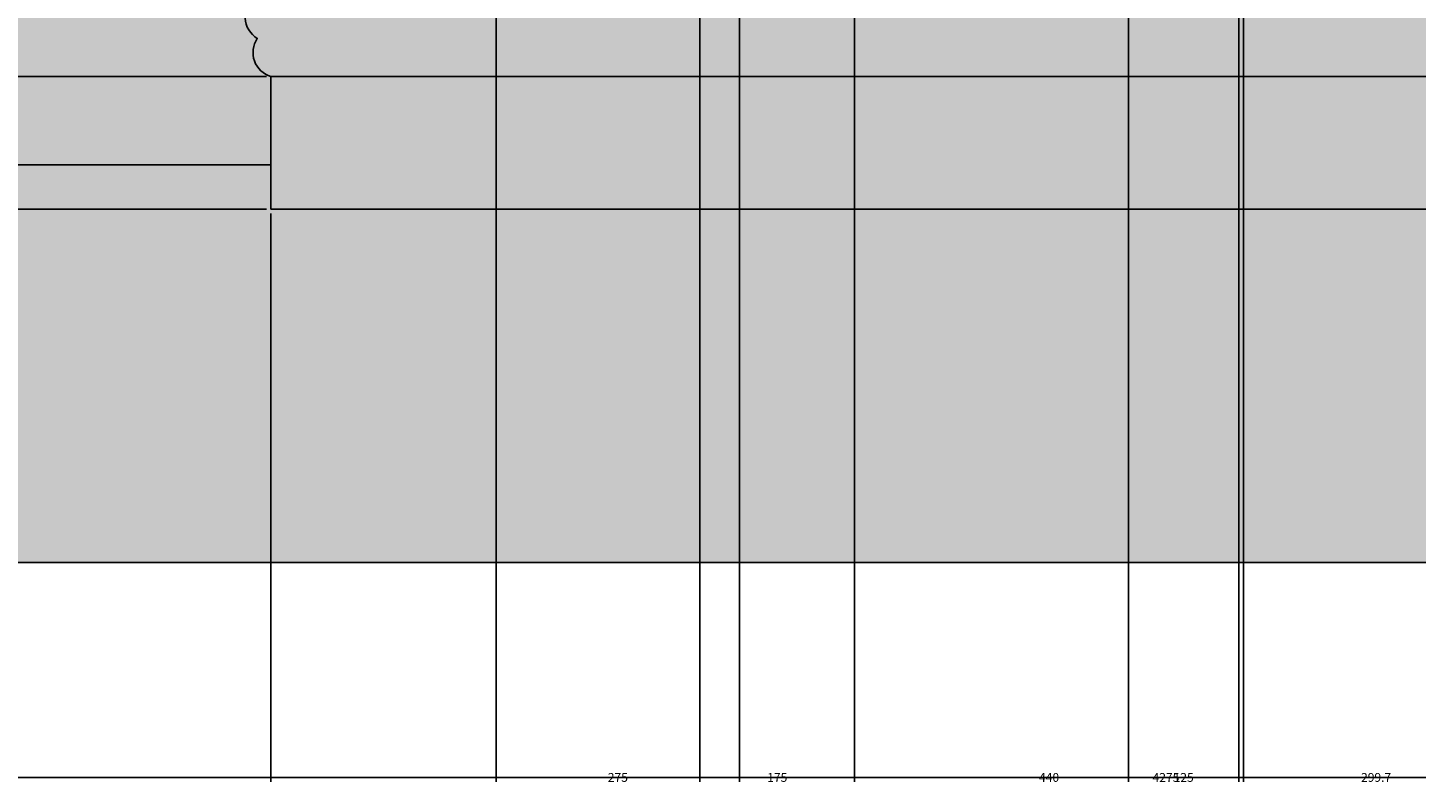
# Model space of a CAD drawing. Units: millimetres. Extents: x 2970 to 7764, y 2196 to 7505.
# Tile 2 of 13: x 4081 to 5651, y 2196 to 3051. Entities that reach past the tile are written whole.
import ezdxf

# ---------------------------------------------------------------- set-up
doc = ezdxf.new("R2010")
doc.units = ezdxf.units.MM
doc.header["$MEASUREMENT"] = 0
for name, color, linetype, lineweight in [('A-ANNO-DIMS', 2, 'Continuous', 18), ('A-ELEV', 7, 'Continuous', 25), ('A-ELEV-PATT', 8, 'Continuous', 13)]:
    doc.layers.add(name, color=color, linetype=linetype, lineweight=lineweight)
doc.styles.get("Standard").update_dxf_attribs({"font": 'arial.ttf'})
doc.dimstyles.get("Standard").update_dxf_attribs({"dimtxt": 10, "dimasz": 5, "dimexe": 5, "dimexo": 5, "dimgap": 2, "dimtad": 0, "dimtih": 1, "dimtoh": 1, "dimdec": 0, "dimzin": 0, "dimdsep": 46, "dimtxsty": 'Standard', "dimcen": 2, "dimadec": 0, "dimazin": 0, "dimtfac": 1, "dimtdec": 0, "dimtofl": 0, "dimtmove": 0, "dimatfit": 3, "dimfxl": 1, "dimtolj": 1, "dimtzin": 0, "dimarcsym": 0})

# ---------------------------------------------------------------- blocks, each defined once
blk = doc.blocks.new('*D10')
at = {"layer": 'A-ANNO-DIMS', "color": 0, "lineweight": -2, "transparency": 16777216}
for p, q in [((3230.5, 2440.8), (3230.5, 2197.8)), ((7505.5, 2440.8), (7505.5, 2197.8)), ((3235.5, 2202.8), (5350.8, 2202.8)), ((7500.5, 2202.8), (5385.2, 2202.8))]:
    blk.add_line(p, q, dxfattribs=at)
at = {"layer": 'A-ANNO-DIMS', "color": 0, "transparency": 16777216}
for points in [[(3235.5, 2203.6), (3235.5, 2202), (3230.5, 2202.8)], [(7500.5, 2203.6), (7500.5, 2202), (7505.5, 2202.8)]]:
    blk.add_solid(points, dxfattribs=at)
at = {"layer": 'Defpoints', "color": 0, "transparency": 16777216}
for p in [(3230.5, 2445.8), (7505.5, 2445.8), (7505.5, 2202.8)]:
    blk.add_point(p, dxfattribs=at)
at = {"layer": 'A-ANNO-DIMS', "color": 0, "transparency": 16777216, "insert": (5368, 2202.8), "char_height": 10, "attachment_point": 5}
blk.add_mtext('\\A1;4275', dxfattribs=at)
blk = doc.blocks.new('*D43')
at = {"layer": 'A-ANNO-DIMS', "color": 0, "lineweight": -2, "transparency": 16777216}
for p, q in [((4355.5, 2840.8), (4355.5, 2197.8)), ((7155.5, 2840.8), (7155.5, 2197.8)), ((4360.5, 2202.8), (5738.5, 2202.8)), ((7150.5, 2202.8), (5772.5, 2202.8))]:
    blk.add_line(p, q, dxfattribs=at)
at = {"layer": 'A-ANNO-DIMS', "color": 0, "transparency": 16777216}
for points in [[(4360.5, 2203.6), (4360.5, 2202), (4355.5, 2202.8)], [(7150.5, 2203.6), (7150.5, 2202), (7155.5, 2202.8)]]:
    blk.add_solid(points, dxfattribs=at)
at = {"layer": 'Defpoints', "color": 0, "transparency": 16777216}
for p in [(4355.5, 2845.8), (7155.5, 2845.8), (7155.5, 2202.8)]:
    blk.add_point(p, dxfattribs=at)
at = {"layer": 'A-ANNO-DIMS', "color": 0, "transparency": 16777216, "insert": (5755.5, 2202.8), "char_height": 10, "attachment_point": 5}
blk.add_mtext('\\A1;2800', dxfattribs=at)
blk = doc.blocks.new('*D44')
at = {"layer": 'A-ANNO-DIMS', "color": 0, "lineweight": -2, "transparency": 16777216}
for p, q in [((4350.5, 2995.8), (2982.5, 2995.8)), ((2987.5, 2990.8), (2987.5, 2927.9)), ((2987.5, 2850.8), (2987.5, 2913.7)), ((4350.5, 2845.8), (2982.5, 2845.8))]:
    blk.add_line(p, q, dxfattribs=at)
at = {"layer": 'A-ANNO-DIMS', "color": 0, "transparency": 16777216}
for points in [[(2986.7, 2990.8), (2988.3, 2990.8), (2987.5, 2995.8)], [(2986.7, 2850.8), (2988.3, 2850.8), (2987.5, 2845.8)]]:
    blk.add_solid(points, dxfattribs=at)
at = {"layer": 'Defpoints', "color": 0, "transparency": 16777216}
for p in [(2987.5, 2995.8), (4355.5, 2995.8), (4355.5, 2845.8)]:
    blk.add_point(p, dxfattribs=at)
at = {"layer": 'A-ANNO-DIMS', "color": 0, "transparency": 16777216, "insert": (2987.5, 2920.8), "char_height": 10, "attachment_point": 5}
blk.add_mtext('\\A1;150', dxfattribs=at)
blk = doc.blocks.new('*D45')
at = {"layer": 'A-ANNO-DIMS', "color": 0, "lineweight": -2, "transparency": 16777216}
for p, q in [((4880.5, 3605.8), (2982.5, 3605.8)), ((2987.5, 3600.8), (2987.5, 3307.9)), ((2987.5, 3000.8), (2987.5, 3293.7)), ((4350.5, 2995.8), (2982.5, 2995.8))]:
    blk.add_line(p, q, dxfattribs=at)
at = {"layer": 'A-ANNO-DIMS', "color": 0, "transparency": 16777216}
for points in [[(2986.7, 3600.8), (2988.3, 3600.8), (2987.5, 3605.8)], [(2986.7, 3000.8), (2988.3, 3000.8), (2987.5, 2995.8)]]:
    blk.add_solid(points, dxfattribs=at)
at = {"layer": 'Defpoints', "color": 0, "transparency": 16777216}
for p in [(2987.5, 3605.8), (4885.5, 3605.8), (4355.5, 2995.8)]:
    blk.add_point(p, dxfattribs=at)
at = {"layer": 'A-ANNO-DIMS', "color": 0, "transparency": 16777216, "insert": (2987.5, 3300.8), "char_height": 10, "attachment_point": 5}
blk.add_mtext('\\A1;610', dxfattribs=at)
blk = doc.blocks.new('*D47')
at = {"layer": 'A-ANNO-DIMS', "color": 0, "lineweight": -2, "transparency": 16777216}
for p, q in [((4610.5, 3613.3), (4610.5, 2197.8)), ((4885.5, 3600.8), (4885.5, 2197.8)), ((4615.5, 2202.8), (4734.8, 2202.8)), ((4880.5, 2202.8), (4761.2, 2202.8))]:
    blk.add_line(p, q, dxfattribs=at)
at = {"layer": 'A-ANNO-DIMS', "color": 0, "transparency": 16777216}
for points in [[(4615.5, 2203.6), (4615.5, 2202), (4610.5, 2202.8)], [(4880.5, 2203.6), (4880.5, 2202), (4885.5, 2202.8)]]:
    blk.add_solid(points, dxfattribs=at)
at = {"layer": 'Defpoints', "color": 0, "transparency": 16777216}
for p in [(4610.5, 3618.3), (4885.5, 3605.8), (4885.5, 2202.8)]:
    blk.add_point(p, dxfattribs=at)
at = {"layer": 'A-ANNO-DIMS', "color": 0, "transparency": 16777216, "insert": (4748, 2202.8), "char_height": 10, "attachment_point": 5}
blk.add_mtext('\\A1;275', dxfattribs=at)
blk = doc.blocks.new('*D48')
at = {"layer": 'A-ANNO-DIMS', "color": 0, "lineweight": -2, "transparency": 16777216}
for p, q in [((5450.5, 3613.3), (5450.5, 2197.8)), ((5325.5, 3600.8), (5325.5, 2197.8)), ((5330.5, 2202.8), (5375.4, 2202.8)), ((5445.5, 2202.8), (5400.6, 2202.8))]:
    blk.add_line(p, q, dxfattribs=at)
at = {"layer": 'A-ANNO-DIMS', "color": 0, "transparency": 16777216}
for points in [[(5330.5, 2203.6), (5330.5, 2202), (5325.5, 2202.8)], [(5445.5, 2203.6), (5445.5, 2202), (5450.5, 2202.8)]]:
    blk.add_solid(points, dxfattribs=at)
at = {"layer": 'Defpoints', "color": 0, "transparency": 16777216}
for p in [(5450.5, 3618.3), (5325.5, 3605.8), (5450.5, 2202.8)]:
    blk.add_point(p, dxfattribs=at)
at = {"layer": 'A-ANNO-DIMS', "color": 0, "transparency": 16777216, "insert": (5388, 2202.8), "char_height": 10, "attachment_point": 5}
blk.add_mtext('\\A1;125', dxfattribs=at)
blk = doc.blocks.new('*D56')
at = {"layer": 'A-ANNO-DIMS', "color": 0, "lineweight": -2, "transparency": 16777216}
for p, q in [((5015.8, 5457.5), (5015.8, 2197.8)), ((5455.8, 5457.5), (5455.8, 2197.8)), ((5020.8, 2202.8), (5222.6, 2202.8)), ((5450.8, 2202.8), (5249, 2202.8))]:
    blk.add_line(p, q, dxfattribs=at)
at = {"layer": 'A-ANNO-DIMS', "color": 0, "transparency": 16777216}
for points in [[(5020.8, 2203.6), (5020.8, 2202), (5015.8, 2202.8)], [(5450.8, 2203.6), (5450.8, 2202), (5455.8, 2202.8)]]:
    blk.add_solid(points, dxfattribs=at)
at = {"layer": 'Defpoints', "color": 0, "transparency": 16777216}
for p in [(5015.8, 5462.5), (5455.8, 5462.5), (5455.8, 2202.8)]:
    blk.add_point(p, dxfattribs=at)
at = {"layer": 'A-ANNO-DIMS', "color": 0, "transparency": 16777216, "insert": (5235.8, 2202.8), "char_height": 10, "attachment_point": 5}
blk.add_mtext('\\A1;440', dxfattribs=at)
blk = doc.blocks.new('*D57')
at = {"layer": 'A-ANNO-DIMS', "color": 0, "lineweight": -2, "transparency": 16777216}
for p, q in [((5455.8, 5457.5), (5455.8, 2197.8)), ((5755.5, 5000.8), (5755.5, 2197.8)), ((5460.8, 2202.8), (5586.7, 2202.8)), ((5750.5, 2202.8), (5624.6, 2202.8))]:
    blk.add_line(p, q, dxfattribs=at)
at = {"layer": 'A-ANNO-DIMS', "color": 0, "transparency": 16777216}
for points in [[(5460.8, 2203.6), (5460.8, 2202), (5455.8, 2202.8)], [(5750.5, 2203.6), (5750.5, 2202), (5755.5, 2202.8)]]:
    blk.add_solid(points, dxfattribs=at)
at = {"layer": 'Defpoints', "color": 0, "transparency": 16777216}
for p in [(5455.8, 5462.5), (5755.5, 5005.8), (5755.5, 2202.8)]:
    blk.add_point(p, dxfattribs=at)
at = {"layer": 'A-ANNO-DIMS', "color": 0, "transparency": 16777216, "insert": (5605.7, 2202.8), "char_height": 10, "attachment_point": 5}
blk.add_mtext('\\A1;299.7', dxfattribs=at)
blk = doc.blocks.new('*D66')
at = {"layer": 'A-ANNO-DIMS', "color": 0, "lineweight": -2, "transparency": 16777216}
for p, q in [((4840.8, 6232.5), (4840.8, 2197.8)), ((5015.8, 6057.5), (5015.8, 2197.8)), ((4845.8, 2202.8), (4915.7, 2202.8)), ((5010.8, 2202.8), (4940.9, 2202.8))]:
    blk.add_line(p, q, dxfattribs=at)
at = {"layer": 'A-ANNO-DIMS', "color": 0, "transparency": 16777216}
for points in [[(4845.8, 2203.6), (4845.8, 2202), (4840.8, 2202.8)], [(5010.8, 2203.6), (5010.8, 2202), (5015.8, 2202.8)]]:
    blk.add_solid(points, dxfattribs=at)
at = {"layer": 'Defpoints', "color": 0, "transparency": 16777216}
for p in [(4840.8, 6237.5), (5015.8, 6062.5), (5015.8, 2202.8)]:
    blk.add_point(p, dxfattribs=at)
at = {"layer": 'A-ANNO-DIMS', "color": 0, "transparency": 16777216, "insert": (4928.3, 2202.8), "char_height": 10, "attachment_point": 5}
blk.add_mtext('\\A1;175', dxfattribs=at)

msp = doc.modelspace()

# ---------------------------------------------------------------- hatches: boundary and pattern name
at = {"layer": 'A-ELEV-PATT'}
h = msp.add_hatch(color=256, dxfattribs=at)
h.set_gradient(color1=(53, 53, 54), color2=(99, 100, 102), name='SPHERICAL')
h.paths.add_polyline_path([(4405.5, 6255.789), (3905.5, 6255.789), (3905.5, 4205.789), (3905.5, 2895.789), (4355.5, 2895.789), (4355.5, 2995.799, -0.50803883), (4340.162, 3038.75, -0.52056705), (4337.177, 3086.472, -0.19797947), (4355.5, 3108.072), (4355.5, 4205.789), (4405.5, 4205.789)])
h.paths.add_polyline_path([(4080.5, 5228.289), (4105.5, 5328.289), (4105.5, 5503.289), (4080.5, 5603.289), (4230.5, 5603.289), (4205.5, 5503.289), (4205.5, 5328.289), (4230.5, 5228.289)], flags=16)
h.paths.add_polyline_path([(4120.5, 5343.289), (4120.5, 5488.289), (4190.5, 5488.289), (4190.5, 5343.289)], flags=0)
h.paths.add_polyline_path([(4230.5, 3923.289), (4205.5, 3823.289), (4205.5, 3648.289), (4230.5, 3548.289), (4080.5, 3548.289), (4105.5, 3648.289), (4105.5, 3823.289), (4080.5, 3923.289)], flags=16)
h.paths.add_polyline_path([(4190.5, 3808.289), (4190.5, 3663.289), (4120.5, 3663.289), (4120.5, 3808.289)], flags=0)
h = msp.add_hatch(color=256, dxfattribs=at)
h.set_gradient(color1=(0, 255, 0), color2=(0, 153, 0), name='INVCURVED')
h.paths.add_polyline_path([(5156.781, 3159.254, 0.52056705), (5077.995, 3099.615, 0.44420267), (4962.635, 3135.756, 0.17969754), (4967.824, 3157.271, 0.6400553), (4827.314, 3199.809, 0.52056705), (4765.24, 3178.339, 0.48686678), (4754.056, 3098.592, -0.0165827), (4758.078, 3094.844, -0.02688608), (4754.056, 3098.592, 0.49967099), (4624.381, 3070.989, 0.37512524), (4571.284, 3103.834, 0.37342356), (4583.794, 3164.025, 0.52056705), (4519.333, 3216.508, 0.52056705), (4438.16, 3192.652, 0.52056705), (4395.384, 3104.368, 0.52056705), (4337.177, 3086.472, 0.52056705), (4340.162, 3038.75, 0.50842605), (4355.534, 2995.789), (5854.747, 2995.789, 0.43666624), (5849.141, 3020.892, 0.52056705), (5873.015, 3051.904, 0.52056705), (5873.015, 3123.471, 0.52056705), (5877.79, 3197.423, 0.52056705), (5865.853, 3228.435, 0.52056705), (5820.491, 3221.279, 0.25799727), (5784.015, 3210.89, 0.32013944), (5748.868, 3259.448, 0.52056705), (5705.894, 3233.206, 0.52056705), (5689.182, 3161.64, 0.44962196), (5599.555, 3145.665, 0.30236269), (5588.909, 3164.025, 0.52056705), (5579.359, 3235.592, 0.52056705), (5498.186, 3233.206, 0.52056705), (5476.699, 3175.953, 0.43983375), (5432.911, 3123.272, 0.4540886), (5352.552, 3152.098, 0.52056705), (5254.666, 3214.122, 0.52056705)])
h = msp.add_hatch(color=256, dxfattribs=at)
h.set_gradient(color1=(76, 66, 38), color2=(0, 0, 0), name='INVSPHERICAL')
h.paths.add_polyline_path([(4355.5, 2995.789), (4355.5, 2895.789), (4355.5, 2845.789), (5855.271, 2845.789), (5855.271, 2995.789)])
h = msp.add_hatch(color=256, dxfattribs=at)
h.dxf.hatch_style = 1
h.paths.add_polyline_path([(7505.5, 2945.789), (7155.5, 2945.789), (7155.5, 2845.789), (6905.5, 2845.789), (4355.5, 2845.789), (4355.5, 2895.789), (3730.5, 2895.789), (3730.5, 2945.789), (3230.5, 2945.789), (3230.5, 2445.789), (7505.5, 2445.789)])

# ---------------------------------------------------------------- linework, layer by layer
at = {"layer": 'A-ELEV'}
for p, q in [((4355.5, 2995.799), (4355.5, 2895.789)), ((4355.5, 2895.789), (4355.5, 2995.789)), ((4355.5, 2995.789), (5855.271, 2995.789)), ((4355.5, 2895.789), (3730.5, 2895.789)), ((4355.5, 2845.789), (4355.5, 2895.789)), ((6905.5, 2845.789), (4355.5, 2845.789)), ((7505.5, 2445.789), (3230.5, 2445.789))]:
    msp.add_line(p, q, dxfattribs=at)
msp.add_lwpolyline([(4355.534, 2995.789, -0.50842605), (4340.162, 3038.75, -0.52056705), (4337.177, 3086.472, -0.52056705), (4395.384, 3104.368, -0.52056705), (4438.16, 3192.652, -0.52056705), (4519.333, 3216.508, -0.52056705), (4583.794, 3164.025, -0.37342356), (4571.284, 3103.834, -0.37342356)], format="xyb", dxfattribs=at)

# ---------------------------------------------------------------- dimensions: what is measured, and where the dimension line sits
at = {"layer": 'A-ANNO-DIMS'}
for base, p1, p2, override, picture, middle in [((5015.81, 2202.789), (4840.81, 6237.49), (5015.81, 6062.49), {"dimdec": 0, "dimlfac": 1, "dimrnd": 0, "dimzin": 0, "dimdsep": 46, "dimlunit": 2}, '*D66', (4928.31, 2202.789)), ((5455.81, 2202.789), (5015.81, 5462.49), (5455.81, 5462.49), {"dimdec": 0, "dimlfac": 1, "dimrnd": 0, "dimzin": 0, "dimdsep": 46, "dimlunit": 2}, '*D56', (5235.81, 2202.789)), ((5755.5, 2202.789), (5455.81, 5462.49), (5755.5, 5005.789), {"dimdec": 1, "dimlfac": 1, "dimrnd": 0, "dimzin": 0, "dimdsep": 46, "dimlunit": 2}, '*D57', (5605.655, 2202.789)), ((4885.5, 2202.789), (4610.5, 3618.289), (4885.5, 3605.789), {"dimdec": 0, "dimlfac": 1, "dimrnd": 0, "dimzin": 0, "dimdsep": 46, "dimlunit": 2}, '*D47', (4748, 2202.789)), ((5450.5, 2202.789), (5325.5, 3605.789), (5450.5, 3618.289), {"dimdec": 0, "dimlfac": 1, "dimrnd": 0, "dimzin": 0, "dimdsep": 46, "dimlunit": 2}, '*D48', (5388, 2202.789)), ((7155.5, 2202.789), (4355.5, 2845.789), (7155.5, 2845.789), {"dimdec": 0, "dimlfac": 1, "dimrnd": 0, "dimzin": 0, "dimdsep": 46, "dimlunit": 2}, '*D43', (5755.5, 2202.789)), ((7505.5, 2202.789), (3230.5, 2445.789), (7505.5, 2445.789), {"dimdec": 0, "dimlfac": 1, "dimrnd": 0, "dimzin": 0, "dimdsep": 46, "dimlunit": 2}, '*D10', (5368, 2202.789))]:
    dim = msp.add_linear_dim(base=base, p1=p1, p2=p2, dimstyle='Standard', override=override, dxfattribs=at)
    dim.commit()
    dim.dimension.update_dxf_attribs({"geometry": picture, "text_midpoint": middle})
for base, p1, p2, picture, middle in [((2987.5, 3605.789), (4355.5, 2995.789), (4885.5, 3605.789), '*D45', (2987.5, 3300.789)), ((2987.5, 2995.789), (4355.5, 2845.789), (4355.5, 2995.789), '*D44', (2987.5, 2920.789))]:
    dim = msp.add_linear_dim(base=base, p1=p1, p2=p2, angle=90, dimstyle='Standard', override={"dimdec": 0, "dimlfac": 1, "dimrnd": 0, "dimzin": 0, "dimdsep": 46, "dimlunit": 2}, dxfattribs=at)
    dim.commit()
    dim.dimension.update_dxf_attribs({"geometry": picture, "text_midpoint": middle})

doc.saveas('drawing.dxf')
